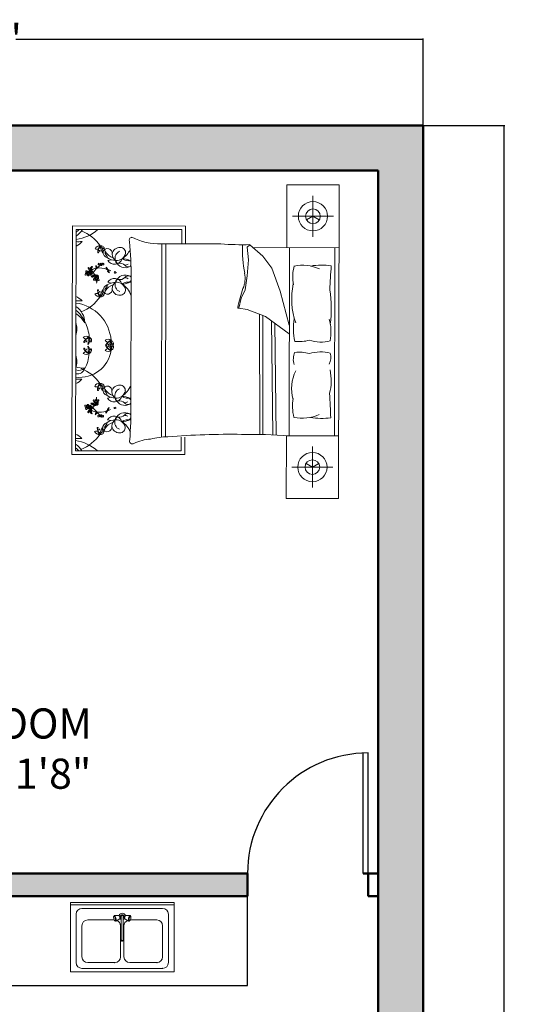
# Model space of a CAD drawing. Units: inches. Extents: x 3 to 485, y -522 to 42.
# Tile 4 of 6: x 132 to 235, y -161 to 35. Entities that reach past the tile are written whole.
import ezdxf

# ---------------------------------------------------------------- set-up
doc = ezdxf.new("R2010")
doc.units = ezdxf.units.IN
doc.header["$MEASUREMENT"] = 0
for name, color, linetype, lineweight in [('A-ANNO-DIMS', 2, 'Continuous', 18), ('A-AREA-IDEN', 7, 'Continuous', 18), ('A-DOOR', 3, 'Continuous', 25), ('A-FLOR-CASE', 8, 'Continuous', 25), ('A-FLOR-FIXT', 9, 'Continuous', 18), ('A-FURN', 8, 'Continuous', 18), ('A-WALL', 7, 'Continuous', 50)]:
    doc.layers.add(name, color=color, linetype=linetype, lineweight=lineweight)
doc.layers.add('A-WALL-PATT', color=18, linetype='Continuous', lineweight=13, true_color=0x000000)
doc.styles.get("Standard").update_dxf_attribs({"font": 'arial.ttf'})
doc.dimstyles.get("Standard").update_dxf_attribs({"dimtxt": 0.18, "dimasz": 0.18, "dimexe": 0.18, "dimexo": 0.0625, "dimgap": 0.09, "dimtad": 0, "dimtih": 1, "dimtoh": 1, "dimdec": 0, "dimzin": 0, "dimdsep": 46, "dimlunit": 3, "dimtxsty": 'Standard', "dimcen": 0.09, "dimadec": 0, "dimazin": 0, "dimtfac": 1, "dimtdec": 0, "dimtofl": 0, "dimtmove": 0, "dimatfit": 3, "dimfxl": 1, "dimtolj": 1, "dimtzin": 0, "dimarcsym": 0})

# ---------------------------------------------------------------- blocks, each defined once
blk = doc.blocks.new('М07 600х900')
for p, q in [((0, 600), (-900, 600)), ((-900, 0), (-900, 600)), ((-900, 0), (-900, 600)), ((0, 0), (0, 600)), ((0, 0), (0, 600)), ((0, 580), (-900, 580)), ((-800, 550), (-100, 550)), ((-850, 80), (-850, 500)), ((-750, 450), (-519.1, 450)), ((-524.9, 472.1), (-524.8, 476.7)), ((-524.3, 466.5), (-524.9, 472.1)), ((-524.8, 476.7), (-523.8, 479.9)), ((-523, 460.4), (-524.3, 466.5)), ((-520.9, 485.6), (-523.8, 479.9)), ((-523.8, 479.9), (-522.2, 481.3)), ((-521.1, 454.5), (-523, 460.4)), ((-522.2, 481.3), (-520.1, 480.9)), ((-518.8, 449.4), (-521.1, 454.5)), ((-520.9, 485.6), (-518.9, 487.4)), ((-520.1, 480.9), (-517.7, 478.6)), ((-479.6, 487.6), (-518.9, 487.4)), ((-518.9, 487.4), (-516.3, 486.8)), ((-516.4, 445.5), (-518.8, 449.4)), ((-517.7, 478.6), (-515.3, 474.7)), ((-514, 443.2), (-516.4, 445.5)), ((-516.3, 486.8), (-513.3, 484)), ((-515.3, 474.7), (-513, 469.5)), ((-508.6, 439.7), (-514, 443.2)), ((-511.9, 442.7), (-514, 443.2)), ((-513.3, 484), (-510.2, 479.1)), ((-513, 469.5), (-511.1, 463.6)), ((-510.3, 444.2), (-511.9, 442.7)), ((-511.1, 463.6), (-509.8, 457.6)), ((-509.4, 447.3), (-510.3, 444.2)), ((-510.2, 479.1), (-507.4, 472.6)), ((-509.8, 457.6), (-509.2, 452)), ((-509.2, 452), (-509.4, 447.3)), ((-506, 439.1), (-508.6, 439.7)), ((-507.4, 472.6), (-505, 465.3)), ((-471.8, 458.6), (-506, 439.1)), ((-504, 440.9), (-506, 439.1)), ((-505, 465.3), (-503.4, 457.7)), ((-502.8, 444.9), (-504, 440.9)), ((-503.4, 457.7), (-502.6, 450.7)), ((-502.6, 450.7), (-502.8, 444.9)), ((-479.6, 487.6), (-478, 487.3)), ((-478, 487.3), (-476.2, 485.5)), ((-477, 486.3), (-476.6, 488.7)), ((-476.6, 488.7), (-472.7, 496.5)), ((-461.4, 489.4), (-476.2, 485.4)), ((-476.2, 485.5), (-474.4, 482.6)), ((-474.4, 482.6), (-472.7, 478.7)), ((-472.7, 496.5), (-466.5, 502.7)), ((-472.7, 478.7), (-471.2, 474.3)), ((-470.6, 459.7), (-471.8, 458.6)), ((-471.2, 474.3), (-470.3, 469.8)), ((-469.9, 462.1), (-470.6, 459.7)), ((-470.3, 469.8), (-469.8, 465.6)), ((-466.5, 457.3), (-470.2, 461.1)), ((-469.8, 465.6), (-469.9, 462.1)), ((-458.5, 465.3), (-469.9, 462.2)), ((-466.5, 502.7), (-458.7, 506.6)), ((-458.7, 453.4), (-466.5, 457.3)), ((-465, 480), (-462.1, 488.8)), ((-462.1, 471.2), (-465, 480)), ((-462.1, 488.8), (-454.6, 494.3)), ((-458.5, 468.5), (-462.1, 471.2)), ((-458.7, 506.6), (-450, 508)), ((-458.5, 453.3), (-458.7, 453.4)), ((-458.5, 480), (-456.9, 485)), ((-458.5, 480), (-458.5, 279.9)), ((-456.9, 485), (-452.6, 488.1)), ((-454.6, 494.3), (-445.4, 494.3)), ((-452.6, 488.1), (-447.4, 488.1)), ((-450, 508), (-441.3, 506.6)), ((-447.4, 488.1), (-443.1, 485)), ((-445.4, 494.3), (-437.9, 488.8)), ((-443.1, 485), (-441.5, 480)), ((-441.5, 480), (-441.5, 279.9)), ((-437.9, 471.2), (-441.5, 468.5)), ((-441.5, 465.3), (-430.1, 462.2)), ((-441.3, 453.4), (-441.5, 453.3)), ((-441.3, 506.6), (-433.5, 502.7)), ((-433.5, 457.3), (-441.3, 453.4)), ((-438.6, 489.4), (-423.8, 485.4)), ((-437.9, 488.8), (-435, 480)), ((-435, 480), (-437.9, 471.2)), ((-433.5, 502.7), (-427.3, 496.5)), ((-429.8, 461.1), (-433.5, 457.3)), ((-430.2, 465.6), (-429.7, 469.8)), ((-430.1, 462.1), (-430.2, 465.6)), ((-429.4, 459.7), (-430.1, 462.1)), ((-429.7, 469.8), (-428.8, 474.3)), ((-428.2, 458.6), (-429.4, 459.7)), ((-428.8, 474.3), (-427.3, 478.7)), ((-428.2, 458.6), (-394, 439.1)), ((-427.3, 496.5), (-423.4, 488.7)), ((-427.3, 478.7), (-425.6, 482.6)), ((-425.6, 482.6), (-423.8, 485.5)), ((-423.8, 485.5), (-422, 487.3)), ((-423.4, 488.7), (-423, 486.3)), ((-422, 487.3), (-420.4, 487.6)), ((-420.4, 487.6), (-381.1, 487.4)), ((-397.4, 450.7), (-396.6, 457.7)), ((-397.2, 444.9), (-397.4, 450.7)), ((-396, 440.9), (-397.2, 444.9)), ((-396.6, 457.7), (-395, 465.3)), ((-394, 439.1), (-396, 440.9)), ((-395, 465.3), (-392.6, 472.6)), ((-391.4, 439.7), (-394, 439.1)), ((-392.6, 472.6), (-389.8, 479.1)), ((-391.4, 439.7), (-386, 443.2)), ((-390.8, 452), (-390.2, 457.6)), ((-390.6, 447.3), (-390.8, 452)), ((-389.7, 444.2), (-390.6, 447.3)), ((-390.2, 457.6), (-388.9, 463.6)), ((-389.8, 479.1), (-386.7, 484)), ((-388.1, 442.7), (-389.7, 444.2)), ((-388.9, 463.6), (-387, 469.5)), ((-386, 443.2), (-388.1, 442.7)), ((-387, 469.5), (-384.7, 474.7)), ((-386.7, 484), (-383.7, 486.8)), ((-383.6, 445.5), (-386, 443.2)), ((-384.7, 474.7), (-382.3, 478.6)), ((-383.7, 486.8), (-381.1, 487.4)), ((-381.2, 449.4), (-383.6, 445.5)), ((-382.3, 478.6), (-379.9, 480.9)), ((-378.9, 454.5), (-381.2, 449.4)), ((-381.1, 487.4), (-379.1, 485.6)), ((-380.9, 450), (-150, 450)), ((-379.9, 480.9), (-377.8, 481.3)), ((-379.1, 485.6), (-376.2, 479.9)), ((-377, 460.4), (-378.9, 454.5)), ((-377.8, 481.3), (-376.2, 479.9)), ((-375.7, 466.5), (-377, 460.4)), ((-376.2, 479.9), (-375.2, 476.7)), ((-375.1, 472.1), (-375.7, 466.5)), ((-375.2, 476.7), (-375.1, 472.1)), ((-50, 500), (-50, 80)), ((-800, 130), (-800, 400)), ((-465, 400), (-465, 130)), ((-435, 130), (-435, 400)), ((-100, 400), (-100, 130)), ((-458.5, 285.6), (-460.5, 279.9)), ((-460.5, 279.9), (-458.5, 274.2)), ((-458.5, 279.9), (-456.9, 275.3)), ((-458.5, 274.2), (-456.9, 269.8)), ((-458.5, 274.2), (-453.2, 270.6)), ((-456.9, 275.3), (-452.6, 272.4)), ((-456.9, 269.8), (-452.6, 266.9)), ((-453.2, 270.6), (-446.8, 270.6)), ((-452.6, 272.4), (-447.4, 272.4)), ((-452.6, 266.9), (-447.4, 266.9)), ((-447.4, 272.4), (-443.1, 275.3)), ((-447.4, 266.9), (-443.1, 269.8)), ((-446.8, 270.6), (-441.5, 274.2)), ((-443.1, 275.3), (-441.5, 279.9)), ((-441.5, 274.2), (-443.1, 269.8)), ((-439.5, 279.9), (-441.5, 285.6)), ((-441.5, 274.2), (-439.5, 279.9)), ((0, 0), (-900, 0)), ((-100, 30), (-800, 30)), ((-515, 80), (-750, 80)), ((-150, 80), (-385, 80))]:
    blk.add_line(p, q)
for centre, start, end in [((-800, 500), 90, 180), ((-100, 500), 0, 90), ((-750, 400), 90, 180), ((-515, 400), 0, 65.88741), ((-385, 400), 114.11259, 180), ((-150, 400), 0, 90), ((-750, 130), 180, 270), ((-515, 130), 270, 0), ((-385, 130), 180, 270), ((-150, 130), 270, 0), ((-800, 80), 180, 270), ((-100, 80), 270, 0)]:
    blk.add_arc(centre, 50, start, end)
for p in [(-515, 80), (-150, 80), (-100, 30)]:
    blk.add_point(p)
blk = doc.blocks.new('*D4')
at = {"layer": 'A-ANNO-DIMS', "color": 0, "lineweight": -2, "transparency": 16777216}
for p, q in [((30.29, 14.07), (30.29, 31.29)), ((30.47, 31.11), (111.43, 31.11)), ((212.61, 31.11), (131.65, 31.11)), ((212.79, 14.07), (212.79, 31.29))]:
    blk.add_line(p, q, dxfattribs=at)
at = {"layer": 'A-ANNO-DIMS', "color": 0, "transparency": 16777216}
for points in [[(30.47, 31.14), (30.47, 31.08), (30.29, 31.11)], [(212.61, 31.14), (212.61, 31.08), (212.79, 31.11)]]:
    blk.add_solid(points, dxfattribs=at)
at = {"layer": 'Defpoints', "color": 0, "transparency": 16777216}
for p in [(212.79, 31.11), (30.29, 14), (212.79, 14)]:
    blk.add_point(p, dxfattribs=at)
at = {"layer": 'A-ANNO-DIMS', "color": 0, "transparency": 16777216, "insert": (121.54, 31.11), "char_height": 6, "attachment_point": 5}
blk.add_mtext('\\A1;15\'-3"', dxfattribs=at)
blk = doc.blocks.new('*D5')
at = {"layer": 'A-ANNO-DIMS', "color": 0, "lineweight": -2, "transparency": 16777216}
for p, q in [((212.85, 14), (229.02, 14)), ((228.84, 13.82), (228.84, -228.64)), ((228.84, -477.32), (228.84, -234.85)), ((212.85, -477.5), (229.02, -477.5))]:
    blk.add_line(p, q, dxfattribs=at)
at = {"layer": 'A-ANNO-DIMS', "color": 0, "transparency": 16777216}
for points in [[(228.81, 13.82), (228.87, 13.82), (228.84, 14)], [(228.81, -477.32), (228.87, -477.32), (228.84, -477.5)]]:
    blk.add_solid(points, dxfattribs=at)
at = {"layer": 'Defpoints', "color": 0, "transparency": 16777216}
for p in [(212.79, 14), (212.79, -477.5), (228.84, -477.5)]:
    blk.add_point(p, dxfattribs=at)
at = {"layer": 'A-ANNO-DIMS', "color": 0, "transparency": 16777216, "insert": (228.84, -231.75), "char_height": 6, "attachment_point": 5}
blk.add_mtext("\\A1;41'", dxfattribs=at)
blk = doc.blocks.new('BED-DOUBLE-WITH-NIGHTSTANDS')
for p, q in [((53.23, 62.45), (53.09, 0)), ((48, 52.14), (48.02, 60.3)), ((43.93, 56.23), (52.09, 56.21)), ((0, 8.8), (0.1, 54.33)), ((0.1, 54.33), (22.6, 54.28)), ((0.82, 53.6), (0.73, 9.52)), ((21.87, 53.56), (0.82, 53.6)), ((21.87, 50.75), (21.87, 53.56)), ((22.6, 54.28), (22.59, 50.74)), ((17.83, 12.23), (17.92, 50.76)), ((18.61, 12.28), (18.7, 50.76)), ((34.9, 50.06), (35.41, 50.56)), ((35.15, 47.53), (34.9, 50.06)), ((35.41, 50.56), (38.06, 48.28)), ((53.2, 49.96), (36.06, 50)), ((43.33, 49.98), (43.25, 12.51)), ((52.32, 12.49), (52.4, 49.96)), ((7.14, 47.43), (7.85, 47.57)), ((34.89, 44.36), (35.15, 47.53)), ((38.06, 48.28), (39.83, 45.87)), ((39.83, 45.87), (41.46, 41.31)), ((11.71, 18.64), (11.77, 44)), ((34.51, 41.58), (34.89, 44.36)), ((7.13, 43.07), (7.84, 42.93)), ((33.74, 39.94), (34.51, 41.58)), ((41.46, 41.31), (43.3, 34.5)), ((33.23, 37.92), (33.74, 39.94)), ((34.88, 37.66), (33.23, 37.92)), ((38.54, 36.26), (34.88, 37.66)), ((37.41, 12.75), (37.36, 36.71)), ((38.05, 12.75), (38.01, 36.46)), ((43.3, 32.83), (38.54, 36.26)), ((40.02, 12.71), (39.75, 35.39)), ((40.66, 12.69), (40.39, 34.92)), ((7.08, 20.02), (7.79, 20.16)), ((7.07, 15.66), (7.78, 15.52)), ((21.78, 9.47), (21.78, 12.22)), ((22.51, 12.21), (22.5, 8.75)), ((47.91, 10.34), (47.89, 2.18)), ((22.5, 8.75), (0, 8.8)), ((0.73, 9.52), (21.78, 9.47)), ((43.82, 6.27), (51.98, 6.25))]:
    blk.add_line(p, q)
for points in [[(42.79, 49.99), (42.82, 62.48), (53.23, 62.45)], [(48.01, 56.22), (46.75, 55.49)], [(48.01, 56.22), (49.27, 55.49)], [(53.12, 12.49), (42.71, 12.51), (42.69, 0.02), (53.09, 0)], [(47.9, 6.26), (46.64, 6.99)], [(47.9, 6.26), (49.17, 6.98)]]:
    blk.add_lwpolyline(points)
for points in [[(29.69, 50.7, 0.001242), (17.84, 50.76, -0.127202), (11.94, 52.03)], [(51.64, 46.38, 0.074897), (47.56, 46.31, -0.472817)], [(47.3, 31.53, 0.14099), (51.46, 31.4, 0.235245)], [(47.29, 28.87, -0.14099), (51.46, 28.98, -0.235245)], [(51.57, 16.08, -0.074897), (47.49, 16.17, 0.472817)], [(19.1, 12.3, 0.056112), (15.67, 11.85, 0.095341), (12.35, 10.98)]]:
    blk.add_lwpolyline(points, format="xyb")
for centre, radius in [((48.01, 56.22), 2.91), ((48.01, 56.22), 1.46), ((3.2, 44.87), 0.159), ((4.87, 43.83), 0.159), ((3.14, 18.23), 0.159), ((4.82, 19.27), 0.159), ((47.9, 6.26), 2.91), ((47.9, 6.26), 1.46)]:
    blk.add_circle(centre, radius)
for centre, radius, start, end in [((-2.1, 57.02), 4.95, 306.1777, 316.3555), ((-1.36, 55.59), 3.97, 303.3358, 329.9857), ((-0.26, 59.68), 8.16, 277.6191, 311.7597), ((-1.1, 45.72), 8.16, 34.2606, 68.4649), ((-0.45, 53.36), 3.32, 292.4288, 318.8287), ((1.35, 62.44), 11.28, 267.2822, 273.526), ((11.98, 51.45), 0.576, 93.8541, 207.2153), ((-53.24, 44.88), 65.02, 359.2174, 5.5628), ((5.45, 49.43), 0.904, 77.5856, 158.9128), ((4.96, 50.34), 0.681, 238.3374, 358.161), ((7.19, 48.96), 2.06, 138.7143, 177.8093), ((5.23, 49.03), 0.101, 177.8093, 11.3575), ((5.28, 49.04), 0.0492, 11.3575, 127.815), ((5.95, 49.72), 0.667, 117.5568, 223.6503), ((5.53, 49.32), 0.0882, 223.6503, 159.5924), ((5.8, 49.66), 0.676, 2.8257, 103.6021), ((11.21, 51.54), 5.71, 192.3914, 207.0565), ((4.88, 49.27), 1.29, 345.3394, 54.1084), ((6.83, 51.04), 1.39, 211.2568, 255.171), ((7.09, 48.86), 0.937, 350.1381, 160.7429), ((7.38, 49.09), 1.17, 175.8431, 254.1786), ((6.08, 49.06), 0.574, 333.8496, 53.1422), ((9.16, 50.72), 2.95, 211.1355, 251.5786), ((9.5, 48.51), 1.49, 84.8189, 172.7598), ((10.06, 47.93), 1.45, 111.456, 201.2962), ((9.65, 48.95), 1.05, 354.3597, 90.9279), ((7.39, 51.7), 4.73, 303.5412, 333.1738), ((33.98, 107.83), 57.28, 265.7035, 271.4271), ((57.53, 49.44), 23.57, 177.326, 191.2133), ((5.82, 47.83), 1.25, 6.0403, 51.4566), ((8.92, 50.74), 3.35, 236.1624, 266.3817), ((8.49, 48.2), 1.55, 209.7826, 343.0078), ((9.83, 48.77), 1.81, 182.2332, 233.9142), ((8.87, 49.27), 1.88, 265.1674, 346.7951), ((9.14, 47.22), 0.388, 167.1782, 285.0212), ((10.18, 45.36), 2.41, 122.5752, 126.2186), ((10.64, 47.96), 1.99, 199.1563, 299.0492), ((11.32, 49.96), 2.59, 238.6959, 279.0295), ((10.18, 45.36), 2.41, 55.6591, 94.6045), ((11.08, 46.76), 0.752, 29.9034, 52.1991), ((3.07, 45.2), 0.314, 157.2827, 261.3127), ((2.9, 45.21), 0.158, 57.924, 135.5009), ((3.06, 45.11), 0.105, 172.7801, 277.0061), ((2.72, 44.92), 0.501, 14.6299, 57.924), ((3.42, 45.05), 0.217, 35.9787, 181.3022), ((3.43, 45.9), 0.178, 124.2279, 214.2664), ((3.69, 45.87), 0.414, 190.1798, 287.0699), ((3.29, 45.22), 0.219, 269.9386, 331.0248), ((3.81, 46.02), 0.481, 176.8442, 248.1654), ((7.25, 48.55), 4.65, 212.5525, 216.2487), ((3.48, 45.07), 0.156, 263.6267, 41.5794), ((3.65, 45.91), 0.184, 216.2487, 291.6289), ((5.27, 43.32), 2.59, 123.8774, 132.3658), ((2.6, 43), 2.77, 63.656, 68.1654), ((4.08, 45.13), 0.441, 128.1949, 208.6903), ((4.09, 45.78), 0.414, 122.6896, 187.2733), ((3.77, 45.61), 0.139, 289.2346, 111.6289), ((3.87, 45.61), 0.139, 221.7444, 44.1387), ((4.5, 45.2), 0.725, 157.1046, 228.9376), ((4.27, 45.72), 0.481, 109.354, 177.5569), ((4.25, 45.44), 0.427, 174.3285, 220.4929), ((1.82, 43.06), 3.11, 30.4181, 49.6921), ((4.01, 46.03), 0.178, 56.7377, 146.7762), ((4.1, 45.83), 0.184, 148.7585, 224.1387), ((3.54, 44.83), 0.513, 339.8782, 40.4929), ((7.92, 43.52), 4.65, 145.0623, 148.7585), ((5.27, 43.32), 2.59, 94.6301, 119.0782), ((10.78, 39.58), 8.53, 132.1153, 142.0485), ((6.49, 46.38), 1.76, 178.2005, 187.0043), ((4.59, 46.14), 0.328, 11.1997, 64.3362), ((5.7, 46.61), 0.987, 190.1329, 210.5301), ((5.04, 46.21), 0.3, 188.2173, 274.161), ((5.3, 46.37), 0.523, 210.5301, 242.5082), ((5.7, 46.82), 1, 218.0842, 226.1812), ((4.95, 45.98), 0.127, 325.6398, 67.3157), ((1.01, 50.24), 5.93, 313.0282, 321.92), ((5.39, 40.75), 5.17, 73.4583, 93.7018), ((5.37, 46.67), 0.122, 142.3478, 264.9271), ((5.53, 46.7), 0.263, 127.6362, 168.9144), ((5.39, 46.92), 0.37, 264.9271, 338.2359), ((5.88, 46.41), 0.483, 113.3017, 137.4845), ((5.82, 46.91), 0.159, 183.1509, 356.5973), ((5.94, 46.62), 0.26, 139.663, 227.5532), ((5.85, 46.53), 0.137, 227.5532, 350.2228), ((5.32, 46.63), 0.521, 352.9593, 15.5912), ((5.67, 46.57), 0.329, 350.2228, 43.5279), ((6.28, 46.9), 0.382, 198.6004, 262.3773), ((5.97, 46.73), 0.152, 0.9822, 91.7416), ((6.07, 46.69), 0.265, 11.4378, 52.5099), ((6.26, 46.64), 0.123, 255.1097, 54.7989), ((8.59, 46), 1.76, 178.2005, 187.0043), ((6.69, 45.76), 0.328, 11.1997, 64.3362), ((7.8, 46.23), 0.987, 190.1329, 210.5301), ((7.14, 45.83), 0.3, 188.2173, 274.161), ((7.4, 46), 0.523, 210.5301, 242.5082), ((7.8, 46.44), 1, 218.0842, 226.1812), ((7.05, 45.6), 0.127, 325.6398, 67.3157), ((7.41, 45.37), 0.3, 147.4073, 233.3509), ((7.68, 45.52), 0.523, 179.06, 211.0381), ((7.17, 45.41), 0.127, 354.2525, 95.9284), ((5.39, 40.75), 5.17, 62.8773, 69.7682), ((8.08, 45.76), 0.987, 211.0381, 231.4353), ((8.25, 46.56), 1.76, 234.5639, 243.3677), ((8.27, 45.66), 1, 195.387, 203.484), ((7.14, 45.01), 0.328, 357.232, 50.3685), ((8.55, 45.07), 0.12, 12.5792, 190.3125), ((8.62, 45.08), 0.196, 190.3125, 10.2877), ((9.57, 45.61), 1.28, 41.4394, 105.0212), ((10.28, 48.26), 1.8, 277.3101, 299.789), ((11.23, 47.07), 0.935, 221.4394, 293.7095), ((11.08, 46.76), 0.752, 314.3258, 333.4321), ((52.37, 44.15), 8.37, 164.978, 190.911), ((45.9, 38.43), 8.05, 65.0057, 101.6324), ((645.92, 10.65), 595.35, 176.55931, 177.02387), ((2.74, 44.63), 0.122, 142.3478, 264.9271), ((2.9, 44.66), 0.263, 61.0937, 168.9144), ((2.76, 44.88), 0.37, 264.9271, 338.2359), ((3.25, 44.37), 0.483, 113.3017, 137.4845), ((3.31, 44.59), 0.26, 139.663, 227.5532), ((3.23, 44.5), 0.137, 227.5532, 350.2228), ((2.7, 44.59), 0.521, 352.9593, 15.5912), ((3.04, 44.53), 0.329, 350.2228, 43.5279), ((3.48, 45.17), 0.25, 221.7153, 265.6618), ((3.65, 44.87), 0.382, 198.6004, 262.3773), ((3.35, 44.69), 0.152, 0.9822, 91.7416), ((3.44, 44.65), 0.265, 11.4378, 86.2391), ((3.63, 44.61), 0.123, 255.1097, 54.7989), ((4.16, 45.16), 0.527, 207.5784, 254.2257), ((3.82, 44.86), 0.725, 270.1521, 341.9851), ((4.3, 43.95), 0.513, 98.5968, 159.2116), ((4.05, 44.61), 0.527, 244.864, 291.5114), ((4.16, 44.88), 0.427, 278.5968, 324.7613), ((4.09, 44.54), 0.441, 290.3994, 358.4116), ((4.41, 43.59), 0.122, 142.3478, 264.9271), ((4.57, 43.61), 0.263, 61.0937, 168.9144), ((4.44, 43.84), 0.37, 264.9271, 338.2359), ((4.75, 44.15), 0.314, 157.2827, 261.3127), ((4.57, 44.17), 0.158, 57.924, 135.5009), ((4.95, 44.66), 0.441, 182.724, 265.9967), ((4.78, 44.97), 0.427, 231.6348, 277.7993), ((5.11, 45.05), 0.725, 214.411, 286.244), ((4.92, 43.33), 0.483, 113.3017, 137.4845), ((4.74, 44.07), 0.105, 172.7801, 277.0061), ((4.39, 43.87), 0.501, 14.6299, 57.924), ((1.82, 43.06), 3.11, 22.9242, 23.7218), ((4.99, 43.54), 0.26, 139.663, 227.5532), ((4.9, 43.45), 0.137, 227.5532, 350.2228), ((4.9, 44.04), 0.513, 37.1845, 97.7993), ((5.09, 44.01), 0.217, 35.9787, 181.3022), ((4.37, 43.55), 0.521, 352.9593, 15.5912), ((4.96, 44.75), 0.527, 264.8847, 311.5321), ((1.82, 43.06), 3.11, 356.9812, 4.6326), ((4.71, 43.48), 0.329, 350.2228, 43.5279), ((5.32, 43.82), 0.382, 198.6004, 262.3773), ((4.97, 44.18), 0.219, 269.9386, 331.0248), ((5.15, 44.12), 0.25, 221.7153, 265.6618), ((5.02, 43.64), 0.152, 0.9822, 91.7416), ((5.15, 44.03), 0.156, 263.6267, 41.5794), ((5.12, 43.61), 0.265, 11.4378, 86.2391), ((5.3, 43.56), 0.123, 255.1097, 54.7989), ((8.48, 42.29), 1.55, 16.7404, 149.9656), ((9.81, 41.72), 1.81, 125.834, 177.515), ((9.13, 43.27), 0.388, 74.727, 192.57), ((10.63, 42.53), 1.99, 60.699, 160.5919), ((10.18, 45.13), 2.41, 233.5296, 237.173), ((9.57, 44.88), 1.28, 254.727, 318.3088), ((10.27, 42.23), 1.8, 59.9592, 82.4381), ((11.22, 43.41), 0.935, 66.0387, 138.3088), ((11.08, 43.73), 0.752, 307.5491, 336.5885), ((11.08, 43.73), 0.752, 23.1031, 45.4224), ((29.42, 43.87), 5.08, 336.1357, 11.2133), ((5.21, 41.48), 0.101, 348.3907, 181.9389), ((7.17, 41.55), 2.06, 181.9389, 221.0339), ((5.26, 41.47), 0.0492, 231.9332, 348.3907), ((5.93, 40.78), 0.667, 136.0979, 242.1914), ((5.55, 41.17), 0.0532, 200.1408, 136.1012), ((4.87, 41.24), 1.29, 305.6398, 14.4087), ((11.19, 38.94), 5.71, 152.6917, 167.3568), ((7.36, 41.41), 1.17, 105.5696, 183.9051), ((7.08, 41.64), 0.937, 199.0053, 9.6101), ((6.06, 41.45), 0.574, 306.606, 25.8985), ((5.81, 42.68), 1.25, 308.2916, 353.7079), ((9.14, 39.78), 2.95, 108.1696, 148.6127), ((8.9, 39.75), 3.35, 93.3665, 123.5858), ((9.48, 41.98), 1.49, 186.9883, 274.9292), ((10.05, 42.56), 1.45, 158.4519, 248.2922), ((8.85, 41.22), 1.88, 12.9531, 94.5808), ((9.63, 41.55), 1.05, 268.8203, 5.3885), ((11.3, 40.52), 2.59, 79.5874, 121.0523), ((10.18, 45.13), 2.41, 265.1437, 304.089), ((7.36, 38.8), 4.73, 21.3682, 56.207), ((56.83, 33.53), 24.22, 159.9935, 169.2124), ((58.3, 39.73), 14.52, 167.9138, 199.1356), ((29.02, 37.87), 22.65, 352.0937, 9.3711), ((-0.49, 37.18), 3.32, 40.9195, 67.3194), ((1.28, 28.09), 11.28, 86.2222, 92.466), ((-1.1, 44.81), 8.16, 291.2833, 325.4876), ((4.94, 40.17), 0.681, 1.5872, 121.4108), ((5.43, 41.08), 0.904, 200.8354, 282.1626), ((5.78, 40.85), 0.676, 256.1461, 356.9225), ((6.81, 39.46), 1.39, 104.5772, 148.4914), ((-0.33, 30.86), 8.16, 4.3364, 82.1291), ((-1.41, 34.95), 3.97, 1.1461, 56.4124), ((-2.15, 33.52), 4.95, 17.7245, 53.5705), ((33.18, 38.06), 0.151, 178.7364, 289.6277), ((-3.55, 30.92), 7.37, 33.8864, 53.9271), ((55.12, 33.86), 11.01, 169.7358, 193.4979), ((40.46, 33.06), 11.13, 351.399, 13.8341), ((-3.51, 33.77), 4.48, 343.4172, 16.8943), ((-4.69, 31.49), 8.16, 4.3364, 27.2887), ((-5.82, 32), 6.63, 4.2528, 5.5098), ((-10.38, 28.52), 11.85, 19.5958, 19.7769), ((2.83, 31.44), 0.904, 47.6614, 128.9886), ((2.86, 32.47), 0.681, 208.4132, 328.2368), ((4.1, 30.16), 2.06, 108.79, 147.8851), ((3.41, 31.44), 0.667, 87.6326, 193.7261), ((2.85, 31.31), 0.0882, 193.7261, 129.7986), ((8.88, 30.39), 5.71, 162.4671, 177.1323), ((2.26, 31.58), 1.29, 315.4152, 24.1842), ((4.83, 32.14), 1.39, 181.3326, 225.2468), ((3.25, 31.46), 0.676, 332.9015, 73.6778), ((7.2, 30.81), 0.904, 47.6614, 128.9886), ((7.23, 31.83), 0.681, 208.4132, 328.2368), ((8.47, 29.52), 2.06, 108.79, 147.8851), ((7.78, 30.81), 0.667, 87.6326, 193.7261), ((6.63, 30.95), 1.29, 315.4152, 24.1842), ((13.25, 29.76), 5.71, 162.4671, 177.1323), ((7.62, 30.83), 0.676, 332.9015, 73.6778), ((9.2, 31.51), 1.39, 181.3326, 225.2468), ((45.23, 38.9), 7.65, 263.887, 285.7034), ((1.56, 30.44), 6.31, 262.7377, 351.6938), ((2.44, 31.2), 0.101, 147.8851, 341.4333), ((2.44, 29.83), 0.101, 18.3149, 211.8631), ((4.1, 30.87), 2.06, 211.8631, 250.9581), ((2.49, 31.18), 0.0492, 341.4333, 97.8908), ((2.49, 29.85), 0.0492, 261.8574, 18.3149), ((3.41, 29.58), 0.667, 166.0221, 272.1156), ((2.88, 29.73), 0.0532, 230.065, 165.895), ((8.88, 30.61), 5.71, 182.6159, 197.2811), ((2.26, 29.45), 1.29, 335.564, 44.333), ((4.82, 28.88), 1.39, 134.5014, 178.4156), ((3.24, 29.57), 0.676, 286.0703, 26.8467), ((7.22, 29.18), 0.681, 31.5114, 151.335), ((7.2, 30.2), 0.904, 230.7596, 312.0868), ((6.81, 30.57), 0.101, 147.8851, 341.4333), ((6.81, 30.45), 0.101, 18.3149, 211.8631), ((8.47, 31.48), 2.06, 211.8631, 250.9581), ((6.86, 30.55), 0.0492, 341.4333, 97.8908), ((6.86, 30.46), 0.0492, 261.8574, 18.3149), ((7.78, 30.2), 0.667, 166.0221, 272.1156), ((7.22, 30.67), 0.0882, 193.7261, 129.7986), ((7.25, 30.35), 0.0532, 230.065, 165.895), ((6.63, 30.06), 1.29, 335.564, 44.333), ((13.25, 31.23), 5.71, 182.6159, 197.2811), ((7.61, 30.18), 0.676, 286.0703, 26.8467), ((9.19, 29.49), 1.39, 134.5014, 178.4156), ((-3.52, 27.29), 4.48, 342.8539, 16.331), ((-5.83, 29.07), 6.63, 354.2384, 355.4954), ((-10.37, 32.57), 11.85, 339.9713, 340.1524), ((2.85, 28.56), 0.681, 31.5114, 151.335), ((2.83, 29.59), 0.904, 230.7596, 312.0868), ((-4.7, 29.57), 8.16, 332.4595, 355.4118), ((47.41, 27.72), 3.31, 154.8924, 198.4148), ((45.19, 21.51), 7.65, 74.0448, 95.8612), ((48.49, 28.13), 3.09, 333.2178, 15.9767), ((2.13, 29.63), 3.65, 247.9911, 276.4936), ((1.11, 26.28), 1.46, 256.2639, 348.9479), ((1.31, 27.38), 1.85, 252.735, 311.779), ((-1.16, 18.31), 8.16, 34.2606, 68.4649), ((40.66, 23.52), 10.98, 346.2168, 11.0582), ((1.29, 35.03), 11.28, 267.2822, 273.526), ((-0.51, 25.95), 3.32, 292.4288, 318.8287), ((51.7, 21.92), 7.95, 153.7502, 196.0487), ((5.39, 22.02), 0.904, 77.5856, 158.9128), ((4.9, 22.93), 0.681, 238.3374, 358.161), ((7.13, 21.54), 2.06, 138.7143, 177.8093), ((5.17, 21.62), 0.101, 177.8093, 11.3575), ((5.22, 21.63), 0.0492, 11.3575, 127.815), ((5.89, 22.31), 0.667, 117.5568, 223.6503), ((5.47, 21.91), 0.0882, 223.6503, 159.5924), ((5.74, 22.25), 0.676, 2.8257, 103.6021), ((6.77, 23.63), 1.39, 211.2568, 255.171), ((4.82, 21.86), 1.29, 345.3394, 54.1084), ((11.15, 24.13), 5.71, 192.3914, 207.0565), ((7.03, 21.45), 0.937, 350.1381, 160.7429), ((7.32, 21.68), 1.17, 175.8431, 254.1786), ((6.02, 21.65), 0.574, 333.8496, 53.1422), ((9.1, 23.31), 2.95, 211.1355, 251.5786), ((9.44, 21.1), 1.49, 84.8189, 172.7598), ((10, 20.52), 1.45, 111.456, 201.2962), ((9.59, 21.54), 1.05, 354.3597, 90.9279), ((7.33, 24.29), 4.73, 303.5412, 338.38), ((4.36, 19.51), 0.122, 94.8211, 217.4004), ((4.38, 19.27), 0.37, 21.5123, 94.8211), ((4.93, 19.56), 0.26, 132.1949, 220.0852), ((4.85, 19.65), 0.137, 9.5254, 132.1949), ((4.32, 19.56), 0.521, 344.157, 6.7889), ((1.77, 20.05), 3.11, 355.1156, 2.767), ((4.66, 19.62), 0.329, 316.2203, 9.5254), ((5.27, 19.28), 0.382, 97.3709, 161.1478), ((5.25, 19.54), 0.123, 304.9493, 104.6385), ((5.76, 20.42), 1.25, 6.0403, 51.4566), ((8.86, 23.33), 3.35, 236.1624, 266.3817), ((8.43, 20.79), 1.55, 209.7826, 343.0078), ((9.77, 21.36), 1.81, 182.2332, 233.9142), ((8.81, 21.86), 1.88, 265.1674, 346.7951), ((9.08, 19.81), 0.388, 167.1782, 285.0212), ((10.12, 17.95), 2.41, 122.5752, 126.2186), ((10.58, 20.55), 1.99, 199.1563, 299.0492), ((11.26, 22.55), 2.59, 238.6959, 280.1608), ((10.12, 17.95), 2.41, 55.6591, 94.6045), ((11.02, 19.35), 0.752, 23.1597, 52.1991), ((52.31, 18.31), 8.37, 168.8372, 194.7702), ((646, 49.2), 595.35, 182.72432, 183.18889), ((2.68, 18.48), 0.122, 94.8211, 217.4004), ((2.84, 18.45), 0.263, 190.8338, 298.6545), ((2.7, 18.23), 0.37, 21.5123, 94.8211), ((3.01, 17.91), 0.314, 98.4355, 202.4655), ((2.84, 17.9), 0.158, 224.2473, 301.8242), ((3.19, 18.73), 0.483, 222.2637, 246.4465), ((3, 18), 0.105, 82.7421, 186.9681), ((2.66, 18.19), 0.501, 301.8242, 345.1183), ((3.25, 18.52), 0.26, 132.1949, 220.0852), ((3.17, 18.61), 0.137, 9.5254, 132.1949), ((2.64, 18.52), 0.521, 344.157, 6.7889), ((3.36, 18.06), 0.217, 178.446, 323.7695), ((2.98, 18.58), 0.329, 316.2203, 9.5254), ((3.59, 18.24), 0.382, 97.3709, 161.1478), ((3.42, 17.94), 0.25, 94.0864, 138.0328), ((3.23, 17.89), 0.219, 28.7234, 89.8096), ((3.29, 18.42), 0.152, 268.0066, 358.766), ((3.38, 18.45), 0.265, 273.5091, 348.3104), ((3.42, 18.03), 0.156, 318.1687, 96.1215), ((5.22, 19.78), 2.59, 227.3824, 235.8708), ((3.57, 18.5), 0.123, 304.9493, 104.6385), ((4.02, 17.97), 0.441, 151.0579, 231.5533), ((4.11, 17.94), 0.527, 105.5225, 152.1698), ((4.44, 17.9), 0.725, 130.8106, 202.6436), ((3.99, 18.49), 0.527, 68.2368, 114.8842), ((3.76, 18.24), 0.725, 17.763, 89.5961), ((4.25, 19.15), 0.513, 200.5366, 261.1514), ((1.77, 20.05), 3.11, 310.0561, 329.3301), ((4.19, 17.66), 0.427, 139.2553, 185.4197), ((3.48, 18.28), 0.513, 319.2553, 19.87), ((10.75, 23.5), 8.53, 217.6997, 227.6329), ((4.1, 18.22), 0.427, 34.9869, 81.1514), ((4.03, 18.57), 0.441, 1.3366, 69.3488), ((4.52, 19.49), 0.263, 190.8338, 298.6545), ((4.69, 18.95), 0.314, 98.4355, 202.4655), ((4.52, 18.94), 0.158, 224.2473, 301.8242), ((4.89, 18.44), 0.441, 93.7515, 177.0242), ((5.05, 18.05), 0.725, 73.5042, 145.3372), ((4.72, 18.13), 0.427, 81.9489, 128.1134), ((4.87, 19.77), 0.483, 222.2637, 246.4465), ((4.68, 19.04), 0.105, 82.7421, 186.9681), ((4.34, 19.23), 0.501, 301.8242, 345.1183), ((1.77, 20.05), 3.11, 336.0264, 336.824), ((4.85, 19.06), 0.513, 261.9489, 322.5636), ((5.04, 19.1), 0.217, 178.446, 323.7695), ((4.9, 18.36), 0.527, 48.2161, 94.8635), ((5.1, 18.98), 0.25, 94.0864, 138.0328), ((4.91, 18.92), 0.219, 28.7234, 89.8096), ((4.97, 19.46), 0.152, 268.0066, 358.766), ((5.06, 19.49), 0.265, 273.5091, 348.3104), ((5.1, 19.07), 0.156, 318.1687, 96.1215), ((7.35, 17.72), 0.3, 126.3973, 212.3409), ((7.62, 17.57), 0.523, 148.7101, 180.6882), ((7.11, 17.69), 0.127, 263.8198, 5.4957), ((5.35, 22.35), 5.17, 289.98, 296.8709), ((8.02, 17.33), 0.987, 128.3129, 148.7101), ((8.19, 16.52), 1.76, 116.3805, 125.1843), ((8.2, 17.43), 1, 156.2642, 164.3612), ((7.08, 18.09), 0.328, 309.3797, 2.5162), ((8.56, 18), 0.196, 349.4605, 169.4356), ((8.49, 18.02), 0.12, 169.4356, 347.169), ((9.51, 18.2), 1.28, 41.4394, 105.0212), ((10.22, 20.85), 1.8, 277.3101, 299.789), ((11.17, 19.66), 0.935, 221.4394, 293.7095), ((-49.04, 16.86), 60.77, 355.1143, 1.6776), ((11.02, 19.35), 0.752, 314.3258, 336.5885), ((3.37, 17.21), 0.178, 145.4818, 235.5203), ((3.63, 17.23), 0.414, 72.6783, 169.5684), ((3.75, 17.09), 0.481, 111.5828, 182.904), ((7.17, 14.54), 4.65, 143.4995, 147.1957), ((3.58, 17.2), 0.184, 68.1193, 143.4995), ((2.55, 20.11), 2.77, 291.5828, 296.0922), ((4.02, 17.33), 0.414, 172.4749, 237.0586), ((3.7, 17.5), 0.139, 248.1193, 70.5136), ((3.81, 17.5), 0.139, 315.6095, 138.0038), ((4.21, 17.38), 0.481, 182.1913, 250.3942), ((3.95, 17.08), 0.178, 212.972, 303.0105), ((4.04, 17.27), 0.184, 135.6095, 210.9897), ((7.86, 19.57), 4.65, 210.9897, 214.6859), ((5.22, 19.78), 2.59, 240.67, 265.1181), ((5.63, 16.49), 0.987, 149.2181, 169.6153), ((6.42, 16.72), 1.76, 172.7439, 181.5477), ((4.52, 16.96), 0.328, 295.412, 348.5485), ((4.97, 16.89), 0.3, 85.5872, 171.5309), ((5.24, 16.73), 0.523, 117.24, 149.2181), ((5.63, 16.28), 1, 133.567, 141.664), ((4.89, 17.12), 0.127, 292.4324, 34.1083), ((5.35, 22.35), 5.17, 266.0464, 286.2899), ((0.93, 12.88), 5.93, 37.8282, 46.72), ((5.3, 16.43), 0.122, 94.8211, 217.4004), ((5.46, 16.4), 0.263, 190.8338, 232.112), ((5.32, 16.18), 0.37, 21.5123, 94.8211), ((5.81, 16.69), 0.483, 222.2637, 246.4465), ((5.75, 16.19), 0.159, 3.1509, 176.5973), ((5.87, 16.47), 0.26, 132.1949, 220.0852), ((5.79, 16.56), 0.137, 9.5254, 132.1949), ((5.26, 16.47), 0.521, 344.157, 6.7889), ((5.6, 16.53), 0.329, 316.2203, 9.5254), ((6.21, 16.19), 0.382, 97.3709, 161.1478), ((5.91, 16.37), 0.152, 268.0066, 358.766), ((6.19, 16.45), 0.123, 304.9493, 104.6385), ((6, 16.41), 0.265, 307.2383, 348.3104), ((8.53, 17.08), 1.76, 172.7439, 181.5477), ((7.74, 16.86), 0.987, 149.2181, 169.6153), ((6.62, 17.33), 0.328, 295.412, 348.5485), ((7.08, 17.26), 0.3, 85.5872, 171.5309), ((7.34, 17.09), 0.523, 117.24, 149.2181), ((7.73, 16.64), 1, 133.567, 141.664), ((6.99, 17.49), 0.127, 292.4324, 34.1083), ((8.42, 14.88), 1.55, 16.7404, 149.9656), ((9.75, 14.31), 1.81, 125.834, 177.515), ((8.79, 13.81), 1.88, 12.9531, 94.5808), ((9.07, 15.86), 0.388, 74.727, 192.57), ((10.57, 15.12), 1.99, 60.699, 160.5919), ((10.12, 17.72), 2.41, 233.5296, 237.173), ((9.51, 17.47), 1.28, 254.727, 318.3088), ((11.24, 13.11), 2.59, 79.1231, 121.0523), ((10.12, 17.72), 2.41, 265.1437, 304.089), ((10.21, 14.82), 1.8, 59.9592, 82.4381), ((11.16, 16), 0.935, 66.0387, 138.3088), ((11.01, 16.32), 0.752, 307.5491, 342.4555), ((11.01, 16.32), 0.752, 16.5084, 45.4224), ((45.87, 24.05), 8.05, 258.1158, 294.7425), ((5.15, 14.07), 0.101, 348.3907, 181.9389), ((7.11, 14.14), 2.06, 181.9389, 221.0339), ((5.2, 14.06), 0.0492, 231.9332, 348.3907), ((5.87, 13.37), 0.667, 136.0979, 242.1914), ((5.49, 13.76), 0.0532, 200.1408, 136.1012), ((11.12, 11.53), 5.71, 152.6917, 167.3568), ((4.81, 13.83), 1.29, 305.6398, 14.4087), ((7.3, 14), 1.17, 105.5696, 183.9051), ((7.02, 14.23), 0.937, 199.0053, 9.6101), ((6, 14.04), 0.574, 306.606, 25.8985), ((5.75, 15.27), 1.25, 308.2916, 353.7079), ((9.08, 12.37), 2.95, 108.1696, 148.6127), ((8.84, 12.34), 3.35, 93.3665, 123.5858), ((9.42, 14.57), 1.49, 186.9883, 274.9292), ((9.99, 15.15), 1.45, 158.4519, 248.2922), ((9.57, 14.14), 1.05, 268.8203, 5.3885), ((7.3, 11.39), 4.73, 23.5194, 56.207), ((-0.55, 9.77), 3.32, 40.9195, 67.3194), ((1.22, 0.68), 11.28, 86.2222, 92.466), ((-1.16, 17.4), 8.16, 291.2833, 325.4876), ((4.88, 12.76), 0.681, 1.5872, 121.4108), ((5.37, 13.67), 0.904, 200.8354, 282.1626), ((6.75, 12.05), 1.39, 104.5772, 148.4914), ((5.72, 13.44), 0.676, 256.1461, 356.9225), ((31.22, -133.58), 146.38, 88.9886, 94.7476), ((35.37, -99.43), 112.22, 85.9741, 90.8023), ((-0.39, 3.45), 8.16, 47.9885, 82.1291), ((-1.47, 7.54), 3.97, 29.7625, 56.4124), ((-2.21, 6.11), 4.95, 43.3927, 53.5705), ((12.04, 11.46), 0.569, 156.396, 303.7005)]:
    blk.add_arc(centre, radius, start, end)
blk = doc.blocks.new('DOOR-SWING-24IN')
for p, q in [((-1, 0), (-1, 24)), ((0, 0), (0, 24))]:
    blk.add_line(p, q)
blk.add_arc((0, 0), 24, 90, 180)

msp = doc.modelspace()

# ---------------------------------------------------------------- hatches: boundary and pattern name
at = {"layer": 'A-WALL-PATT'}
h = msp.add_hatch(color=256, dxfattribs=at)
h.dxf.hatch_style = 1
h.paths.add_polyline_path([(177.79, -240), (177.79, -235.5), (39.29, -235.5), (39.29, 5), (87.29, 5), (87.29, -53), (91.79, -53), (91.79, 5), (203.79, 5), (203.79, -477.5), (212.79, -477.5), (212.79, 14), (30.29, 14), (30.29, -477.5), (39.29, -477.5), (39.29, -388.5), (94.55, -388.5), (94.55, -384), (39.29, -384), (39.29, -240)])
h.paths.add_polyline_path([(142.75, -477.5), (142.75, -468.5), (82.75, -468.5), (82.75, -477.5)], flags=17)
h.paths.add_polyline_path([(63.29, -79), (63.29, -83.5), (87.29, -83.5), (89.54, -83.5), (91.79, -83.5), (91.79, -77), (87.29, -77), (87.29, -79)], flags=17)
h.paths.add_polyline_path([(177.79, -139.5), (177.79, -135), (91.79, -135), (87.29, -135), (87.29, -139.5), (91.79, -139.5)], flags=17)

# ---------------------------------------------------------------- linework, layer by layer
at = {"layer": 'A-FLOR-CASE'}
for p, q in [((177.79, -157.31), (177.79, -139.5)), ((87.29, -157.31), (177.79, -157.31))]:
    msp.add_line(p, q, dxfattribs=at)
at = {"layer": 'A-WALL'}
for p, q in [((30.29, 14), (212.79, 14)), ((212.79, 14), (212.79, -477.5)), ((91.79, 5), (203.79, 5)), ((203.79, 5), (203.79, -477.5)), ((91.79, -135), (177.79, -135)), ((177.79, -139.5), (177.79, -135)), ((200.79, -135), (203.79, -135)), ((201.79, -135), (201.79, -139.5)), ((91.79, -139.5), (177.79, -139.5)), ((201.79, -139.5), (203.79, -139.5))]:
    msp.add_line(p, q, dxfattribs=at)

# ---------------------------------------------------------------- block references
at = {"layer": 'A-DOOR'}
msp.add_blockref('DOOR-SWING-24IN', (201.79, -135), dxfattribs=at)
at = {"layer": 'A-FLOR-FIXT', "xscale": 0.0229615710193718, "yscale": 0.0229615710193718, "zscale": 0.0229615710193718}
msp.add_blockref('М07 600х900', (163.17, -154.59), dxfattribs=at)
at = {"layer": 'A-FURN'}
msp.add_blockref('BED-DOUBLE-WITH-NIGHTSTANDS', (142.81, -60.33), dxfattribs=at)

# ---------------------------------------------------------------- texts
at = {"layer": 'A-AREA-IDEN', "insert": (106.96, -102.13), "char_height": 6, "attachment_point": 1}
msp.add_mtext('BEDROOM\\P9\'4"X11\'8"', dxfattribs=at)

# ---------------------------------------------------------------- dimensions: what is measured, and where the dimension line sits
at = {"layer": 'A-ANNO-DIMS'}
dim = msp.add_linear_dim(base=(212.79082571, 31.10517539), p1=(30.29082571, 14.00352841), p2=(212.79082571, 14.00352841), dimstyle='Standard', override={"dimtxt": 6, "dimclrd": 0, "dimclre": 0, "dimclrt": 0}, dxfattribs=at)
dim.commit()
dim.dimension.update_dxf_attribs({"geometry": '*D4', "text_midpoint": (121.54082571, 31.10517539)})
dim = msp.add_linear_dim(base=(228.83525514, -477.49647159), p1=(212.79082571, 14.00352841), p2=(212.79082571, -477.49647159), angle=90, dimstyle='Standard', override={"dimtxt": 6, "dimclrd": 0, "dimclre": 0, "dimclrt": 0}, dxfattribs=at)
dim.commit()
dim.dimension.update_dxf_attribs({"geometry": '*D5', "text_midpoint": (228.83525514, -231.74647159)})

doc.saveas('drawing.dxf')
